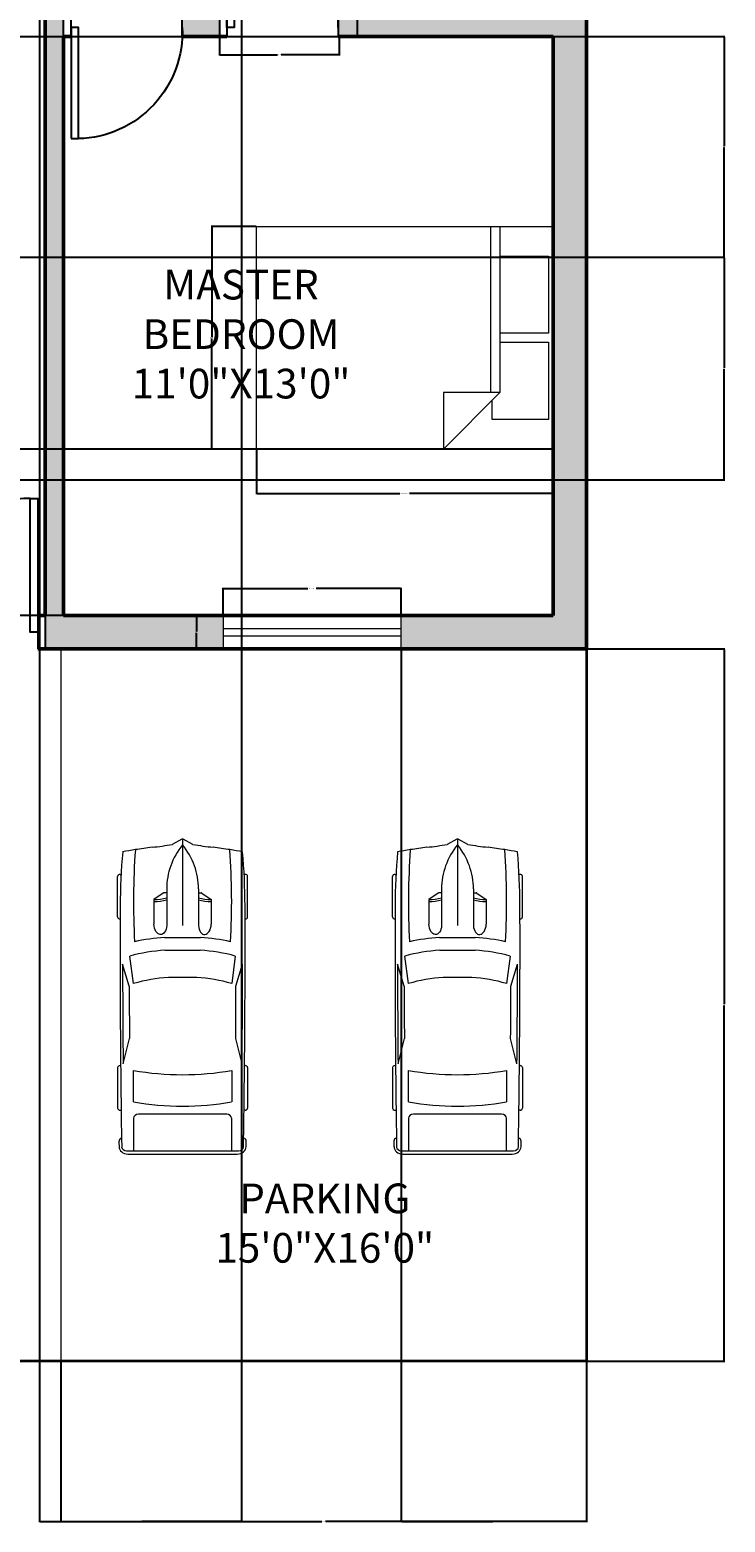
# Model space of a CAD drawing. Units: inches. Extents: x 76 to 532, y 199 to 998.
# Tile 2 of 4: x 345 to 532, y 199 to 601. Entities that reach past the tile are written whole.
import ezdxf

# ---------------------------------------------------------------- set-up
doc = ezdxf.new("R2010")
doc.units = ezdxf.units.IN
for name, color, linetype, lineweight in [('A-ANNO-DIMS', 2, 'Continuous', 18), ('A-AREA-IDEN', 3, 'Continuous', 18), ('A-FURN', 8, 'Continuous', 18), ('A-WALL', 7, 'Continuous', 50), ('A-WALL-PATT', 45, 'Continuous', 13), ('C-PKNG-VEHI', 9, 'Continuous', 13), ('C-PROP', 7, 'Continuous', 35), ('C-SITE', 7, 'Continuous', 18), ('doors', 1, 'Continuous', 25), ('windows', 140, 'Continuous', 18)]:
    doc.layers.add(name, color=color, linetype=linetype, lineweight=lineweight)
doc.styles.get("Standard").update_dxf_attribs({"font": 'arial.ttf'})
doc.dimstyles.get("Standard").update_dxf_attribs({"dimtxt": 0.18, "dimasz": 0.18, "dimexe": 0.18, "dimexo": 0.0625, "dimgap": 0.09, "dimtad": 0, "dimtih": 1, "dimtoh": 1, "dimdec": 4, "dimzin": 0, "dimdsep": 46, "dimtxsty": 'Standard', "dimcen": 0.09, "dimadec": 0, "dimazin": 0, "dimtfac": 1, "dimtdec": 4, "dimtofl": 0, "dimtmove": 0, "dimatfit": 3, "dimfxl": 1, "dimtolj": 1, "dimtzin": 0, "dimarcsym": 0})

# ---------------------------------------------------------------- blocks, each defined once
blk = doc.blocks.new('*U11')
for p, q in [((536, 950), (536, 936)), ((1182, 988), (568, 988)), ((1214, 950), (1214, 950)), ((2235, 810), (1899, 912)), ((3440, 942), (3440, 950)), ((3472, 988), (4087, 988)), ((4119, 950), (4119, 934)), ((1779, 801), (2195, 746)), ((3412, 904), (3030, 807)), ((3516, 746), (3994, 746)), ((4736, 746), (4242, 746)), ((4736, -851), (4736, 851)), ((4785, -832), (4785, 832)), ((4179, 670), (4179, -670)), ((756, 241), (1313, 241)), ((816, 241), (816, 283)), ((820, 295), (918, 436)), ((918, 436), (1294, 436)), ((1496, -274), (1496, 274)), ((1690, -267), (1690, 267)), ((4736, -267), (4736, 267)), ((83, 156), (3, 10)), ((2102, 216), (2102, -216)), ((0, 0), (1313, 0)), ((3, -10), (83, -156)), ((756, -241), (1313, -241)), ((816, -241), (816, -283)), ((820, -295), (918, -436)), ((918, -436), (1294, -436)), ((2195, -746), (1779, -801)), ((2235, -810), (1899, -912)), ((3412, -904), (3030, -807)), ((3994, -746), (3516, -746)), ((4242, -746), (4736, -746)), ((536, -950), (536, -936)), ((1182, -988), (568, -988)), ((1214, -950), (1214, -950)), ((3440, -942), (3440, -950)), ((3472, -988), (4087, -988)), ((4119, -950), (4119, -934))]:
    blk.add_line(p, q)
for centre, major_axis, ratio, start_param, end_param in [((6757, -699), (0, 7958), 0.842304, 1.367076, 1.39176), ((1046, -12468), (0, 13417), 0.842304, 0.00281, 0.075598), ((568, 950), (0, -37.6), 0.842304, 3.141593, 4.712389), ((1638, -268113), (0, 269063), 0.842304, -0.013397, 0.002797), ((1182, 950), (0, 37.6), 0.842304, -1.570796, 0), ((1638, -268113), (0, -269025), 0.842304, 3.133765, 3.140441), ((3472, 950), (0, -37.6), 0.842304, 3.141593, 4.712389), ((4087, 950), (0, 37.6), 0.842304, -1.570796, 0), ((4588, 910), (0, 56.4), 0.842304, -0.013017, 1.249894), ((1638, -268131), (0, 269121), 0.842304, -0.013397, -0.013017), ((4673, 851), (0, -75.2), 0.842304, 1.570796, 3.128196), ((4673, 832), (0, -133), 0.842304, 1.570796, 3.128196), ((6583, -699), (0, -7755), 0.842304, 4.528606, 4.561838), ((952, -15087), (0, -15833), 0.842304, 3.096046, 3.200911), ((3414, 137), (0, -2280), 0.842304, 4.449482, 4.652344), ((3436, 137), (0, 2077), 0.842304, 1.245306, 1.50788), ((3800, 71), (0, -2021), 0.842304, 4.372215, 4.640744), ((2433, -93125), (0, -93935), 0.842304, 3.134049, 3.144098), ((434, 0), (0, 3734), 0.842304, 4.511394, 4.913384), ((912, 0), (0, 3734), 0.842304, 4.511394, 4.913384), ((4242, 670), (0, 75.2), 0.842304, 0, 1.570796), ((-5194, 1331), (0, -6374), 0.842304, 1.385369, 1.434372), ((756, -1185), (0, 1427), 0.842304, 0, 0.590319), ((832, 283), (0, 18.8), 0.842304, 0.879714, 1.570796), ((331, 432), (0, 696), 0.842304, 4.435146, 4.718221), ((361, 432), (0, 696), 0.842304, 4.435146, 4.718221), ((1290, 339), (161, -9), 0.603834, -1.395552, 1.581315), ((16, 0), (0, -18.8), 0.842304, 4.131459, 5.293319), ((-5194, -1331), (0, 6374), 0.842304, -1.434372, -1.385369), ((756, 1185), (0, 1427), 0.842304, 2.551274, 3.141593), ((3800, -71), (0, -2021), 0.842304, -1.499151, -1.230623), ((832, -283), (0, -18.8), 0.842304, 4.712389, 5.403472), ((331, -432), (0, -696), 0.842304, 1.564964, 1.848039), ((361, -432), (0, -696), 0.842304, 1.564964, 1.848039), ((3414, -137), (0, -2280), 0.842304, -1.510751, -1.307889), ((3436, -137), (0, -2077), 0.842304, -1.50788, -1.245306), ((6583, 699), (0, 7755), 0.842304, 1.721348, 1.754579), ((4242, -670), (0, -75.2), 0.842304, 4.712389, 6.283185), ((6757, 699), (0, 7958), 0.842304, 1.749832, 1.774517), ((952, 15087), (0, -15833), 0.842304, -0.059319, 0.045547), ((1638, 268113), (0, -269025), 0.842304, 0.001152, 0.007828), ((2433, 93125), (0, -93935), 0.842304, -0.002505, 0.007544), ((4673, -851), (0, 75.2), 0.842304, 3.15499, 4.712389), ((4673, -832), (0, -133), 0.842304, 0.013397, 1.570796), ((1046, 12468), (0, -13417), 0.842304, -0.075598, -0.00281), ((568, -950), (0, 37.6), 0.842304, 1.570796, 3.141593), ((1638, 268113), (0, 269063), 0.842304, 3.138796, 3.15499), ((1182, -950), (0, -37.6), 0.842304, 0, 1.570796), ((3472, -950), (0, -37.6), 0.842304, -1.570796, 0), ((4087, -950), (0, 37.6), 0.842304, 3.141593, 4.712389), ((4588, -910), (0, -56.4), 0.842304, -1.249894, 0.013017), ((1638, 268131), (0, 269121), 0.842304, 3.15461, 3.15499)]:
    blk.add_ellipse(centre, major_axis=major_axis, ratio=ratio, start_param=start_param, end_param=end_param)
at = {"extrusion": (0, 0, -1)}
blk.add_ellipse((1290, -339), major_axis=(161, 9), ratio=0.603834, start_param=-1.395552, end_param=1.581315, dxfattribs=at)
blk = doc.blocks.new('Bed - Queen')
for p, q in [((0, -80.00003), (0, 0)), ((0, 0), (59.99999, 0)), ((59.99999, 0), (59.99999, -80.00003)), ((7.99999, -1.2), (28.79998, -1.2)), ((7.99999, -14.4), (7.99999, -1.2)), ((28.79998, -1.2), (28.79998, -14.4)), ((31.19999, -1.2), (51.99999, -1.2)), ((31.19999, -14.4), (31.19999, -1.2)), ((51.99999, -1.2), (51.99999, -16.4)), ((0, -14.4), (44.8, -14.4)), ((59.99999, -29.6), (44.8, -14.4)), ((44.8, -14.4), (44.8, -29.6)), ((44.8, -16.8), (0, -16.8)), ((51.99999, -16.4), (46.79936, -16.4)), ((44.8, -29.6), (59.99999, -29.6)), ((59.99999, -80.00003), (0, -80.00003))]:
    blk.add_line(p, q)
blk = doc.blocks.new('DOOR-SWING-30IN')
for p, q in [((0, 5), (0, 0)), ((2, 5), (2, 0)), ((32, 5), (32, 0))]:
    blk.add_line(p, q)
blk.add_lwpolyline([(2, 32.5), (4, 32.5), (4, 2.5), (2, 2.5)], close=True)
blk.add_arc((3.27, 3.75), 28.76, 357.5089, 88.5412)
blk = doc.blocks.new('WIN-48IN')
for p, q in [((0, 5.5), (48, 5.5)), ((0, 3.5), (48, 3.5))]:
    blk.add_line(p, q)
blk.add_lwpolyline([(0, 0), (48, 0), (48, 9), (0, 9)], close=True)
blk = doc.blocks.new('*D15')
at = {"layer": 'A-ANNO-DIMS', "color": 0, "lineweight": -2, "transparency": 16777216}
for p, q in [((428.25, 631.53), (433.25, 631.53)), ((433.07, 631.35), (433.07, 615.46)), ((433.07, 599.21), (433.07, 615.09)), ((428.25, 599.03), (433.25, 599.03))]:
    blk.add_line(p, q, dxfattribs=at)
at = {"layer": 'A-ANNO-DIMS', "color": 0, "transparency": 16777216}
for points in [[(433.04, 631.35), (433.1, 631.35), (433.07, 631.53)], [(433.04, 599.21), (433.1, 599.21), (433.07, 599.03)]]:
    blk.add_solid(points, dxfattribs=at)
at = {"layer": 'Defpoints', "color": 0, "transparency": 16777216}
for p in [(428.19, 631.53), (433.07, 631.53), (428.19, 599.03)]:
    blk.add_point(p, dxfattribs=at)
at = {"layer": 'A-ANNO-DIMS', "color": 0, "transparency": 16777216, "insert": (433.07, 615.28), "char_height": 0.18, "attachment_point": 5}
blk.add_mtext('\\A1;DOOR 33 TYP.', dxfattribs=at)
blk = doc.blocks.new('*D16')
at = {"layer": 'A-ANNO-DIMS', "color": 0, "lineweight": -2, "transparency": 16777216}
for p, q in [((395.86, 598.97), (395.86, 593.97)), ((428.19, 598.97), (428.19, 593.97)), ((396.04, 594.15), (411.5, 594.15)), ((428.01, 594.15), (412.55, 594.15))]:
    blk.add_line(p, q, dxfattribs=at)
at = {"layer": 'A-ANNO-DIMS', "color": 0, "transparency": 16777216}
for points in [[(396.04, 594.18), (396.04, 594.12), (395.86, 594.15)], [(428.01, 594.18), (428.01, 594.12), (428.19, 594.15)]]:
    blk.add_solid(points, dxfattribs=at)
at = {"layer": 'Defpoints', "color": 0, "transparency": 16777216}
for p in [(395.86, 599.03), (428.19, 599.03), (428.19, 594.15)]:
    blk.add_point(p, dxfattribs=at)
at = {"layer": 'A-ANNO-DIMS', "color": 0, "transparency": 16777216, "insert": (412.02, 594.15), "char_height": 0.18, "attachment_point": 5}
blk.add_mtext('\\A1;32 TYP.', dxfattribs=at)
blk = doc.blocks.new('*D17')
at = {"layer": 'A-ANNO-DIMS', "color": 0, "lineweight": -2, "transparency": 16777216}
for p, q in [((396.86, 443.09), (396.86, 450.41)), ((397.04, 450.23), (419.74, 450.23)), ((444.68, 450.23), (421.98, 450.23)), ((444.86, 443.09), (444.86, 450.41))]:
    blk.add_line(p, q, dxfattribs=at)
at = {"layer": 'A-ANNO-DIMS', "color": 0, "transparency": 16777216}
for points in [[(397.04, 450.26), (397.04, 450.2), (396.86, 450.23)], [(444.68, 450.26), (444.68, 450.2), (444.86, 450.23)]]:
    blk.add_solid(points, dxfattribs=at)
at = {"layer": 'Defpoints', "color": 0, "transparency": 16777216}
for p in [(444.86, 450.23), (396.86, 443.03), (444.86, 443.03)]:
    blk.add_point(p, dxfattribs=at)
at = {"layer": 'A-ANNO-DIMS', "color": 0, "transparency": 16777216, "insert": (420.86, 450.23), "char_height": 0.18, "attachment_point": 5}
blk.add_mtext('\\A1;WINDOW 48 TYP.', dxfattribs=at)
blk = doc.blocks.new('*D18')
at = {"layer": 'A-ANNO-DIMS', "color": 0, "lineweight": -2, "transparency": 16777216}
for p, q in [((396.79, 443.03), (389.48, 443.03)), ((389.66, 442.85), (389.66, 438.71)), ((389.66, 434.21), (389.66, 438.35)), ((396.79, 434.03), (389.48, 434.03))]:
    blk.add_line(p, q, dxfattribs=at)
at = {"layer": 'A-ANNO-DIMS', "color": 0, "transparency": 16777216}
for points in [[(389.63, 442.85), (389.69, 442.85), (389.66, 443.03)], [(389.63, 434.21), (389.69, 434.21), (389.66, 434.03)]]:
    blk.add_solid(points, dxfattribs=at)
at = {"layer": 'Defpoints', "color": 0, "transparency": 16777216}
for p in [(389.66, 443.03), (396.86, 443.03), (396.86, 434.03)]:
    blk.add_point(p, dxfattribs=at)
at = {"layer": 'A-ANNO-DIMS', "color": 0, "transparency": 16777216, "insert": (389.66, 438.53), "char_height": 0.18, "attachment_point": 5}
blk.add_mtext('\\A1;9 TYP.', dxfattribs=at)
blk = doc.blocks.new('*D21')
at = {"layer": 'A-ANNO-DIMS', "color": 0, "lineweight": -2, "transparency": 16777216}
for p, q in [((405.86, 487.8), (405.86, 475.68)), ((485.86, 487.8), (485.86, 475.68)), ((406.04, 475.86), (444.55, 475.86)), ((485.68, 475.86), (447.16, 475.86))]:
    blk.add_line(p, q, dxfattribs=at)
at = {"layer": 'A-ANNO-DIMS', "color": 0, "transparency": 16777216}
for points in [[(406.04, 475.89), (406.04, 475.83), (405.86, 475.86)], [(485.68, 475.89), (485.68, 475.83), (485.86, 475.86)]]:
    blk.add_solid(points, dxfattribs=at)
at = {"layer": 'Defpoints', "color": 0, "transparency": 16777216}
for p in [(405.86, 487.86), (485.86, 487.86), (485.86, 475.86)]:
    blk.add_point(p, dxfattribs=at)
at = {"layer": 'A-ANNO-DIMS', "color": 0, "transparency": 16777216, "insert": (445.86, 475.86), "char_height": 0.18, "attachment_point": 5}
blk.add_mtext('\\A1;QUEEN BED 80 TYP.', dxfattribs=at)
blk = doc.blocks.new('*D22')
at = {"layer": 'A-ANNO-DIMS', "color": 0, "lineweight": -2, "transparency": 16777216}
for p, q in [((405.79, 547.86), (393.68, 547.86)), ((393.86, 547.68), (393.86, 518.04)), ((393.86, 488.04), (393.86, 517.68)), ((405.79, 487.86), (393.68, 487.86))]:
    blk.add_line(p, q, dxfattribs=at)
at = {"layer": 'A-ANNO-DIMS', "color": 0, "transparency": 16777216}
for points in [[(393.83, 547.68), (393.89, 547.68), (393.86, 547.86)], [(393.83, 488.04), (393.89, 488.04), (393.86, 487.86)]]:
    blk.add_solid(points, dxfattribs=at)
at = {"layer": 'Defpoints', "color": 0, "transparency": 16777216}
for p in [(405.86, 547.86), (393.86, 487.86), (405.86, 487.86)]:
    blk.add_point(p, dxfattribs=at)
at = {"layer": 'A-ANNO-DIMS', "color": 0, "transparency": 16777216, "insert": (393.86, 517.86), "char_height": 0.18, "attachment_point": 5}
blk.add_mtext('\\A1;60 TYP.', dxfattribs=at)
blk = doc.blocks.new('*D37')
at = {"layer": 'A-ANNO-DIMS', "color": 0, "lineweight": -2, "transparency": 16777216}
for p, q in [((494.92, 434.03), (532.14, 434.03)), ((531.96, 433.85), (531.96, 338.21)), ((531.96, 242.21), (531.96, 337.85)), ((494.92, 242.03), (532.14, 242.03))]:
    blk.add_line(p, q, dxfattribs=at)
at = {"layer": 'A-ANNO-DIMS', "color": 0, "transparency": 16777216}
for points in [[(531.93, 433.85), (531.99, 433.85), (531.96, 434.03)], [(531.93, 242.21), (531.99, 242.21), (531.96, 242.03)]]:
    blk.add_solid(points, dxfattribs=at)
at = {"layer": 'Defpoints', "color": 0, "transparency": 16777216}
for p in [(494.86, 434.03), (531.96, 434.03), (494.86, 242.03)]:
    blk.add_point(p, dxfattribs=at)
at = {"layer": 'A-ANNO-DIMS', "color": 0, "transparency": 16777216, "insert": (531.96, 338.03), "char_height": 0.18, "attachment_point": 5}
blk.add_mtext('\\A1;192', dxfattribs=at)
blk = doc.blocks.new('*D38')
at = {"layer": 'A-ANNO-DIMS', "color": 0, "lineweight": -2, "transparency": 16777216}
for p, q in [((444.86, 433.97), (444.86, 198.6)), ((494.86, 433.97), (494.86, 198.6)), ((445.04, 198.78), (469.64, 198.78)), ((494.68, 198.78), (470.08, 198.78))]:
    blk.add_line(p, q, dxfattribs=at)
at = {"layer": 'A-ANNO-DIMS', "color": 0, "transparency": 16777216}
for points in [[(445.04, 198.81), (445.04, 198.75), (444.86, 198.78)], [(494.68, 198.81), (494.68, 198.75), (494.86, 198.78)]]:
    blk.add_solid(points, dxfattribs=at)
at = {"layer": 'Defpoints', "color": 0, "transparency": 16777216}
for p in [(444.86, 434.03), (494.86, 434.03), (494.86, 198.78)]:
    blk.add_point(p, dxfattribs=at)
at = {"layer": 'A-ANNO-DIMS', "color": 0, "transparency": 16777216, "insert": (469.86, 198.78), "char_height": 0.18, "attachment_point": 5}
blk.add_mtext('\\A1;50', dxfattribs=at)
blk = doc.blocks.new('*D41')
at = {"layer": 'A-ANNO-DIMS', "color": 0, "lineweight": -2, "transparency": 16777216}
for p, q in [((347.36, 900.97), (347.36, 198.6)), ((401.86, 900.97), (401.86, 198.6)), ((347.54, 198.78), (374.28, 198.78)), ((401.68, 198.78), (374.93, 198.78))]:
    blk.add_line(p, q, dxfattribs=at)
at = {"layer": 'A-ANNO-DIMS', "color": 0, "transparency": 16777216}
for points in [[(347.54, 198.81), (347.54, 198.75), (347.36, 198.78)], [(401.68, 198.81), (401.68, 198.75), (401.86, 198.78)]]:
    blk.add_solid(points, dxfattribs=at)
at = {"layer": 'Defpoints', "color": 0, "transparency": 16777216}
for p in [(347.36, 901.03), (401.86, 901.03), (401.86, 198.78)]:
    blk.add_point(p, dxfattribs=at)
at = {"layer": 'A-ANNO-DIMS', "color": 0, "transparency": 16777216, "insert": (374.61, 198.78), "char_height": 0.18, "attachment_point": 5}
blk.add_mtext('\\A1;54.5', dxfattribs=at)
blk = doc.blocks.new('*D43')
at = {"layer": 'A-ANNO-DIMS', "color": 0, "lineweight": -2, "transparency": 16777216}
for p, q in [((353.11, 241.97), (353.11, 198.6)), ((494.86, 241.97), (494.86, 198.6)), ((353.29, 198.78), (423.53, 198.78)), ((494.68, 198.78), (424.44, 198.78))]:
    blk.add_line(p, q, dxfattribs=at)
at = {"layer": 'A-ANNO-DIMS', "color": 0, "transparency": 16777216}
for points in [[(353.29, 198.81), (353.29, 198.75), (353.11, 198.78)], [(494.68, 198.81), (494.68, 198.75), (494.86, 198.78)]]:
    blk.add_solid(points, dxfattribs=at)
at = {"layer": 'Defpoints', "color": 0, "transparency": 16777216}
for p in [(353.11, 242.03), (494.86, 242.03), (494.86, 198.78)]:
    blk.add_point(p, dxfattribs=at)
at = {"layer": 'A-ANNO-DIMS', "color": 0, "transparency": 16777216, "insert": (423.98, 198.78), "char_height": 0.18, "attachment_point": 5}
blk.add_mtext('\\A1;141.74', dxfattribs=at)
blk = doc.blocks.new('*D44')
at = {"layer": 'A-ANNO-DIMS', "color": 0, "lineweight": -2, "transparency": 16777216}
for p, q in [((169.92, 539.57), (532.14, 539.57)), ((531.96, 539.39), (531.96, 509.75)), ((531.96, 479.75), (531.96, 509.39)), ((169.92, 479.57), (532.14, 479.57))]:
    blk.add_line(p, q, dxfattribs=at)
at = {"layer": 'A-ANNO-DIMS', "color": 0, "transparency": 16777216}
for points in [[(531.93, 539.39), (531.99, 539.39), (531.96, 539.57)], [(531.93, 479.75), (531.99, 479.75), (531.96, 479.57)]]:
    blk.add_solid(points, dxfattribs=at)
at = {"layer": 'Defpoints', "color": 0, "transparency": 16777216}
for p in [(169.86, 539.57), (531.96, 539.57), (169.86, 479.57)]:
    blk.add_point(p, dxfattribs=at)
at = {"layer": 'A-ANNO-DIMS', "color": 0, "transparency": 16777216, "insert": (531.96, 509.57), "char_height": 0.18, "attachment_point": 5}
blk.add_mtext('\\A1;60', dxfattribs=at)
blk = doc.blocks.new('*D45')
at = {"layer": 'A-ANNO-DIMS', "color": 0, "lineweight": -2, "transparency": 16777216}
for p, q in [((169.92, 599.03), (532.14, 599.03)), ((531.96, 598.85), (531.96, 569.48)), ((531.96, 539.75), (531.96, 569.12)), ((169.92, 539.57), (532.14, 539.57))]:
    blk.add_line(p, q, dxfattribs=at)
at = {"layer": 'A-ANNO-DIMS', "color": 0, "transparency": 16777216}
for points in [[(531.93, 598.85), (531.99, 598.85), (531.96, 599.03)], [(531.93, 539.75), (531.99, 539.75), (531.96, 539.57)]]:
    blk.add_solid(points, dxfattribs=at)
at = {"layer": 'Defpoints', "color": 0, "transparency": 16777216}
for p in [(169.86, 599.03), (531.96, 599.03), (169.86, 539.57)]:
    blk.add_point(p, dxfattribs=at)
at = {"layer": 'A-ANNO-DIMS', "color": 0, "transparency": 16777216, "insert": (531.96, 569.3), "char_height": 0.18, "attachment_point": 5}
blk.add_mtext('\\A1;59.46', dxfattribs=at)
blk = doc.blocks.new('*D54')
at = {"layer": 'A-ANNO-DIMS', "color": 0, "lineweight": -2, "transparency": 16777216}
for p, q in [((485.79, 487.86), (123.58, 487.86)), ((123.76, 487.68), (123.76, 465.62)), ((123.76, 443.21), (123.76, 465.26)), ((485.79, 443.03), (123.58, 443.03))]:
    blk.add_line(p, q, dxfattribs=at)
at = {"layer": 'A-ANNO-DIMS', "color": 0, "transparency": 16777216}
for points in [[(123.73, 487.68), (123.79, 487.68), (123.76, 487.86)], [(123.73, 443.21), (123.79, 443.21), (123.76, 443.03)]]:
    blk.add_solid(points, dxfattribs=at)
at = {"layer": 'Defpoints', "color": 0, "transparency": 16777216}
for p in [(123.76, 487.86), (485.86, 487.86), (485.86, 443.03)]:
    blk.add_point(p, dxfattribs=at)
at = {"layer": 'A-ANNO-DIMS', "color": 0, "transparency": 16777216, "insert": (123.76, 465.44), "char_height": 0.18, "attachment_point": 5}
blk.add_mtext('\\A1;44.83', dxfattribs=at)

msp = doc.modelspace()

# ---------------------------------------------------------------- hatches: boundary and pattern name
at = {"layer": 'A-WALL-PATT'}
h = msp.add_hatch(color=256, dxfattribs=at)
h.dxf.hatch_style = 1
h.paths.add_polyline_path([(323.3571, 910.0275), (259.8571, 910.0275), (259.8571, 901.0275), (301.8571, 901.0275), (301.8571, 769.0275), (301.8571, 764.0275), (306.8571, 764.0275), (306.8571, 806.0275), (306.8571, 811.0275), (306.8571, 901.0275), (323.3571, 901.0275)])
h.paths.add_polyline_path([(211.8571, 910.0275), (160.8571, 910.0275), (160.8571, 539.5719), (169.8571, 539.5719), (169.8571, 599.0275), (263.8571, 599.0275), (263.8571, 604.0275), (169.8571, 604.0275), (169.8571, 764.0275), (263.8571, 764.0275), (263.8571, 766.5275, -0.0179874), (263.8571, 769.0275), (169.8571, 769.0275), (169.8571, 901.0275), (211.8571, 901.0275)])
h.paths.add_polyline_path([(401.8571, 910.0275), (347.3571, 910.0275), (347.3571, 901.0275), (360.8571, 901.0275), (360.8571, 811.0275), (338.8571, 811.0275, -0.02174236), (338.8571, 808.5275), (338.8571, 806.0275), (360.8571, 806.0275), (360.8571, 764.0275), (365.8571, 764.0275), (365.8571, 836.0275), (397.3621, 836.0275), (397.3621, 841.0275), (365.8571, 841.0275), (365.8571, 901.0275), (401.8571, 901.0275)])
h.paths.add_polyline_path([(169.8571, 479.5719), (160.8571, 479.5719), (160.8571, 434.0275), (211.8571, 434.0275), (211.8571, 443.0275), (169.8571, 443.0275)])
h.paths.add_polyline_path([(310.8571, 443.0275), (259.8571, 443.0275), (259.8571, 434.0275), (310.8571, 434.0275), (310.8571, 438.5275, -0.03336892)])
h.paths.add_polyline_path([(353.8571, 599.0275), (353.8571, 604.0275), (348.8571, 604.0275), (348.8571, 599.0275), (348.8571, 443.0275), (348.8571, 434.0275), (396.8571, 434.0275), (396.8571, 443.0275), (353.8571, 443.0275)])
h.paths.add_polyline_path([(494.8571, 619.5776), (485.8571, 619.5776), (485.8571, 604.0275), (427.8571, 604.0275, -0.02174236), (427.8571, 601.5275), (427.8571, 599.0275), (485.8571, 599.0275), (485.8571, 443.0275), (444.8571, 443.0275), (444.8571, 434.0275), (494.8571, 434.0275)])
h.paths.add_polyline_path([(494.8571, 673.4729), (485.8571, 673.4729), (485.8571, 663.0275), (431.8571, 663.0275), (431.8571, 711.0275), (431.8571, 716.0275), (426.8571, 716.0275), (426.8571, 663.0275), (390.8571, 663.0275), (390.8571, 604.0275), (385.8571, 604.0275), (385.8571, 601.5275, -0.02174236), (385.8571, 599.0275), (395.8571, 599.0275), (395.8571, 604.0275), (395.8571, 658.0275), (430.3571, 658.0275), (430.3571, 659.0275), (451.3571, 659.0275), (451.3571, 658.0275), (485.8571, 658.0275), (485.8571, 643.5776), (494.8571, 643.5776)])
h.paths.add_polyline_path([(494.8571, 752.0275), (485.8571, 752.0275), (485.8571, 716.0275), (463.8571, 716.0275), (463.8571, 713.5275, -0.02174236), (463.8571, 711.0275), (485.8571, 711.0275), (485.8571, 697.4729), (494.8571, 697.4729)])
h.paths.add_polyline_path([(494.8571, 910.0275), (449.8571, 910.0275), (449.8571, 901.0275), (485.8571, 901.0275), (485.8571, 841.0275), (429.3621, 841.0275, -0.02174236), (429.3621, 838.5275), (429.3621, 836.0275), (485.8571, 836.0275), (485.8571, 800.0275), (494.8571, 800.0275)])

# ---------------------------------------------------------------- linework, layer by layer
at = {"layer": 'A-WALL'}
for p, q in [((494.8571, 910.0275), (494.8571, 434.0275)), ((348.8571, 599.0275), (348.8571, 604.0275)), ((348.8571, 599.0275), (348.8571, 443.0275)), ((353.8571, 599.0275), (353.8571, 443.0275)), ((355.8571, 599.0275), (353.8571, 599.0275)), ((397.8571, 599.0275), (385.8571, 599.0275)), ((485.8571, 599.0275), (427.8571, 599.0275)), ((485.8571, 599.0275), (485.8571, 443.0275)), ((348.8571, 443.0275), (346.8571, 443.0275)), ((485.8571, 443.0275), (353.8571, 443.0275)), ((494.8571, 434.0275), (346.8571, 434.0275))]:
    msp.add_line(p, q, dxfattribs=at)
at = {"layer": 'C-PROP'}
for p, q in [((494.8571, 434.0275), (494.8571, 242.0275)), ((494.8571, 242.0275), (160.8571, 242.0275))]:
    msp.add_line(p, q, dxfattribs=at)
at = {"layer": 'C-SITE'}
msp.add_line((353.1127, 434.0275), (353.1127, 242.0275), dxfattribs=at)
at = {"layer": 'doors'}
for p, q in [((346.8571, 443.0275), (346.8571, 434.0275)), ((348.8571, 443.0275), (348.8571, 434.0275))]:
    msp.add_line(p, q, dxfattribs=at)
msp.add_lwpolyline([(344.8571, 474.5275), (346.8571, 474.5275), (346.8571, 438.5275), (344.8571, 438.5275)], close=True, dxfattribs=at)
msp.add_arc((344.5335, 440.7775), 33.7516, 89.450776, 183.822378, dxfattribs=at)

# ---------------------------------------------------------------- block references
at = {"layer": 'A-FURN', "rotation": 270}
msp.add_blockref('Bed - Queen', (485.8571, 547.8578), dxfattribs=at)
at = {"layer": 'C-PKNG-VEHI', "xscale": 0.0177442258840758, "yscale": 0.0177442258840758, "zscale": 0.0177442258840758, "rotation": 270}
for p in [(385.9373, 382.7296), (460.0805, 382.7296)]:
    msp.add_blockref('*U11', p, dxfattribs=at)
at = {"layer": 'doors'}
msp.add_blockref('DOOR-SWING-30IN', (395.8571, 599.0275), dxfattribs=at)
at = {"layer": 'doors', "extrusion": (0, 0, -1), "zscale": -1, "rotation": 180}
msp.add_blockref('DOOR-SWING-30IN', (-353.8571, 604.0275), dxfattribs=at)
at = {"layer": 'windows'}
msp.add_blockref('WIN-48IN', (396.8571, 434.0275), dxfattribs=at)

# ---------------------------------------------------------------- texts
at = {"layer": 'A-AREA-IDEN', "char_height": 8, "attachment_point": 1}
for s, insert in [('\\pxqc;MASTER BEDROOM\\P11\'0"X13\'0"', (361.4045, 536.1722)), ('\\pxqc;PARKING\\P15\'0"X16\'0"', (383.9864, 289.8793))]:
    msp.add_mtext_dynamic_manual_height_columns(s, width=80.600486, gutter_width=12.5, heights=[0], dxfattribs=dict(at, insert=insert))

# ---------------------------------------------------------------- dimensions: what is measured, and where the dimension line sits
at = {"layer": 'A-ANNO-DIMS'}
for base, p1, p2, override, picture, middle in [((401.8571, 198.779), (347.3571, 901.0275), (401.8571, 901.0275), {"dimdec": 1, "dimlfac": 1, "dimrnd": 0, "dimzin": 0, "dimdsep": 46, "dimlunit": 2}, '*D41', (374.6071, 198.779)), ((494.8571, 198.779), (444.8571, 434.0275), (494.8571, 434.0275), {"dimdec": 0, "dimlfac": 1, "dimrnd": 0, "dimzin": 0, "dimdsep": 46, "dimlunit": 2}, '*D38', (469.8571, 198.779)), ((494.8571, 198.779), (353.1127, 242.0275), (494.8571, 242.0275), {"dimdec": 2, "dimlfac": 1, "dimrnd": 0, "dimzin": 0, "dimdsep": 46, "dimlunit": 2}, '*D43', (423.9849, 198.779))]:
    dim = msp.add_linear_dim(base=base, p1=p1, p2=p2, dimstyle='Standard', override=override, dxfattribs=at)
    dim.commit()
    dim.dimension.update_dxf_attribs({"geometry": picture, "text_midpoint": middle})
for base, p1, p2, angle, text, picture, middle in [((433.0674774554, 631.5275074289), (428.1924774554, 599.0275074289), (428.1924774554, 631.5275074289), 90, 'DOOR <> TYP.', '*D15', (433.0674774554, 615.2775074289)), ((393.857, 487.8578), (405.857, 547.8578), (405.857, 487.8578), 270, '<> TYP.', '*D22', (393.857, 517.8578)), ((389.6571, 443.0275), (396.8571, 434.0275), (396.8571, 443.0275), 90, '<> TYP.', '*D18', (389.6571, 438.5275))]:
    dim = msp.add_linear_dim(base=base, p1=p1, p2=p2, angle=angle, text=text, dimstyle='Standard', override={"dimdec": 0, "dimlfac": 1, "dimrnd": 0, "dimzin": 0, "dimdsep": 46, "dimlunit": 2}, dxfattribs=at)
    dim.commit()
    dim.dimension.update_dxf_attribs({"geometry": picture, "text_midpoint": middle})
for base, p1, p2, override, picture, middle in [((531.9571, 599.0275), (169.8571, 539.5719), (169.8571, 599.0275), {"dimdec": 2, "dimlfac": 1, "dimrnd": 0, "dimzin": 0, "dimdsep": 46, "dimlunit": 2}, '*D45', (531.9571, 569.2997)), ((531.9571, 539.5719), (169.8571, 479.5719), (169.8571, 539.5719), {"dimdec": 0, "dimlfac": 1, "dimrnd": 0, "dimzin": 0, "dimdsep": 46, "dimlunit": 2}, '*D44', (531.9571, 509.5719)), ((123.7571, 487.8578), (485.8571, 443.0275), (485.8571, 487.8578), {"dimdec": 2, "dimlfac": 1, "dimrnd": 0, "dimzin": 0, "dimdsep": 46, "dimlunit": 2}, '*D54', (123.7571, 465.4426)), ((531.9571, 434.0275), (494.8571, 242.0275), (494.8571, 434.0275), {"dimdec": 0, "dimlfac": 1, "dimrnd": 0, "dimzin": 0, "dimdsep": 46, "dimlunit": 2}, '*D37', (531.9571, 338.0275))]:
    dim = msp.add_linear_dim(base=base, p1=p1, p2=p2, angle=90, dimstyle='Standard', override=override, dxfattribs=at)
    dim.commit()
    dim.dimension.update_dxf_attribs({"geometry": picture, "text_midpoint": middle})
for base, p1, p2, text, picture, middle in [((428.1925, 594.1525), (395.8571, 599.0275), (428.1925, 599.0275), '<> TYP.', '*D16', (412.0248, 594.1525)), ((485.8571, 475.8578), (405.857, 487.8578), (485.8571, 487.8578), 'QUEEN BED <> TYP.', '*D21', (445.857, 475.8578)), ((444.8571, 450.2275), (396.8571, 443.0275), (444.8571, 443.0275), 'WINDOW <> TYP.', '*D17', (420.8571, 450.2275))]:
    dim = msp.add_linear_dim(base=base, p1=p1, p2=p2, text=text, dimstyle='Standard', override={"dimdec": 0, "dimlfac": 1, "dimrnd": 0, "dimzin": 0, "dimdsep": 46, "dimlunit": 2}, dxfattribs=at)
    dim.commit()
    dim.dimension.update_dxf_attribs({"geometry": picture, "text_midpoint": middle})

doc.saveas('drawing.dxf')
